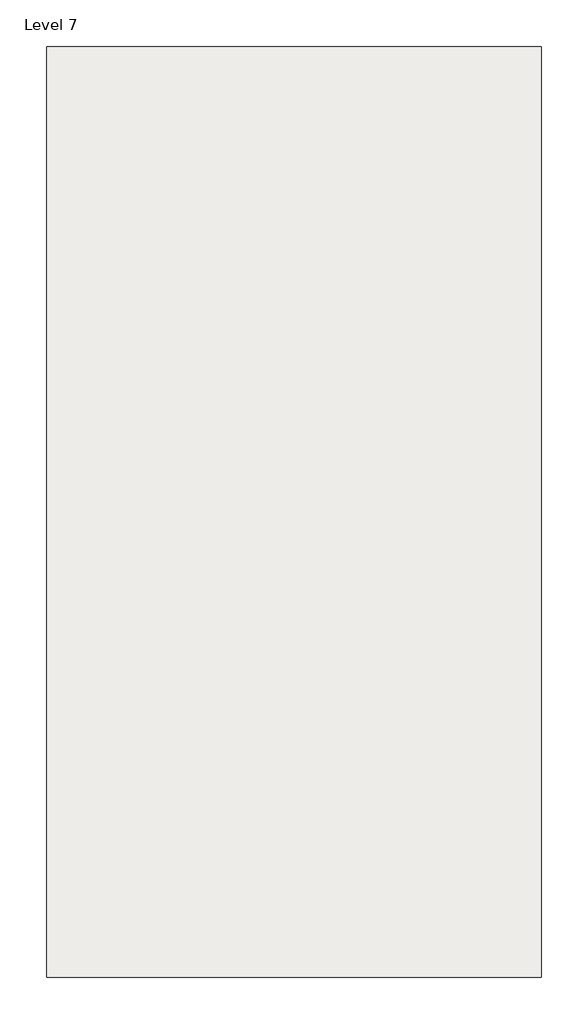
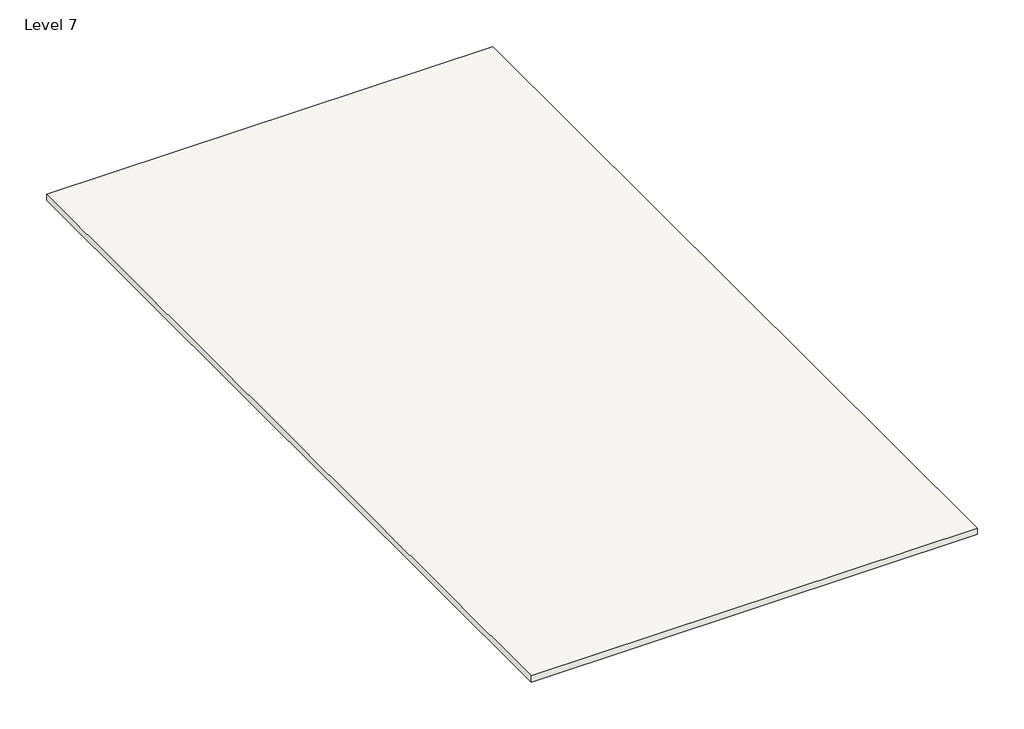
# One storey, incomplete: 1 roof.
"""IFC4 building model written with IfcOpenShell, lengths in millimetres."""

from ifc_helpers import new_model, si_unit, frame, origin, place, context, project, spatial, polyline, outline, extrude, element, save

model = new_model("IFC4")

# Units and contexts
model_context = context("Model", 3, world=origin())
ifc_project = project(units=[si_unit("LENGTHUNIT", "METRE", prefix="MILLI")], contexts=[model_context])

# Site, building, storey
site = spatial("IfcSite", under=ifc_project)
building = spatial("IfcBuilding", under=site)
storey = spatial("IfcBuildingStorey", under=building, Name="Level 7", Elevation=16002.0)

# Roof
placement = place(None, origin())
element("IfcRoof", 1, ObjectType="Generic - 12\"", at=placement, inside=storey, context=model_context, shape_type="SweptSolid", body=[
    extrude(outline(polyline([(-6436.8415084, 11036.6572267), (3926.3584916, 11036.6572267), (3926.3584916, -8470.5427733), (-6436.8415084, -8470.5427733), (-6436.8415084, 11036.6572267)])), frame((0.0, 0.0, 15849.6), z_axis=(0.0, 0.0, 1.0), x_axis=(1.0, 0.0, 0.0)), (0.0, 0.0, 1.0), 152.4),
])

save(model, "model.ifc")

# Revit data of these elements
# Type "Generic - 12\""
#   Assembly Code = "B1020"
#   Layers, outside or top first: 0' - 6" no material (function 1)
# Element 1 (IfcRoof, "Generic - 12\"")
#   built-in parameter 1001705 = 52.5 (stored number, unit not read)
#   built-in parameter 1001701 = -0.5 (stored number, unit not read)
#   built-in parameter 1001710 = 33615
#   Phase Created = New Construction
#   Materials on its faces: "Default Roof", "Wood Planks"
# Materials
#   "Default Roof": colour RGB 88 101 114, transparency 0, Cost = 0
#   "Wood Planks": class "Wood", colour RGB 193 160 115, transparency 0, Description = "Physical material.", Cost = 0
